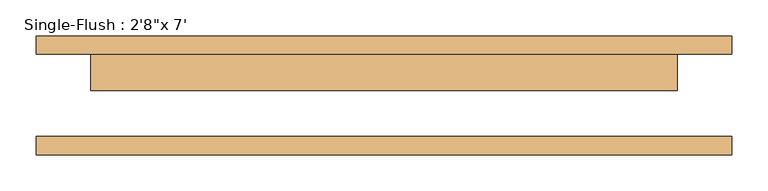
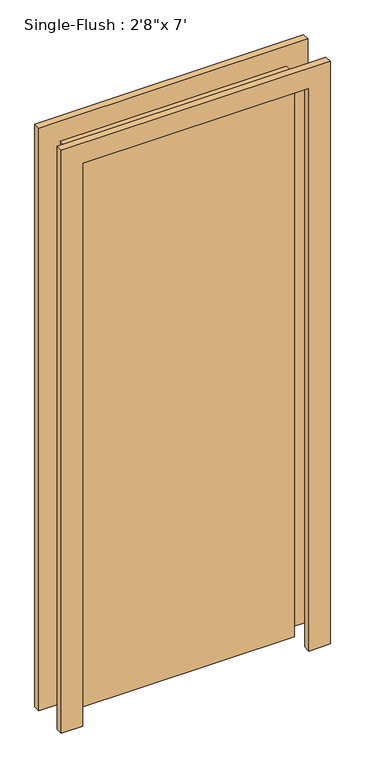
"""IFC4 building model written with IfcOpenShell, lengths in millimetres: door geometry."""

from ifc_helpers import new_model, si_unit, frame, origin, origin_with_axes, place, context, project, spatial, polyline, outline, extrude, source, transform, mapped, element, save


def door_d141acb4(model_context):
    return source(origin(), model_context, "Body", "SweptSolid", [
        extrude(outline(polyline([(2209.8, -482.6), (0.0, -482.6), (0.0, -406.4), (2133.6, -406.4), (2133.6, 406.4), (0.0, 406.4), (0.0, 482.6), (2209.8, 482.6), (2209.8, -482.6)])), frame((0.0, 57.15, 0.0), z_axis=(0.0, 1.0, 0.0), x_axis=(0.0, 0.0, 1.0)), (0.0, 0.0, 1.0), 25.4),
        extrude(outline(polyline([(2209.8, 482.6), (2209.8, -482.6), (0.0, -482.6), (0.0, -406.4), (2133.6, -406.4), (2133.6, 406.4), (0.0, 406.4), (0.0, 482.6), (2209.8, 482.6)])), frame((0.0, -82.55, 0.0), z_axis=(0.0, 1.0, 0.0), x_axis=(0.0, 0.0, 1.0)), (0.0, 0.0, 1.0), 25.4),
        extrude(outline(polyline([(406.4, 6.35), (-406.4, 6.35), (-406.4, 57.15), (406.4, 57.15), (406.4, 6.35)])), origin_with_axes(), (0.0, 0.0, 1.0), 2133.6),
    ])


if __name__ == "__main__":
    model = new_model("IFC4")
    model_context = context("Model", 3, world=origin())
    ifc_project = project(units=[si_unit("LENGTHUNIT", "METRE", prefix="MILLI")], contexts=[model_context])
    site = spatial("IfcSite", under=ifc_project)
    building = spatial("IfcBuilding", under=site)
    placement = place(None, origin())
    door_shape = door_d141acb4(model_context)
    element("IfcDoor", 1, ObjectType="Single-Flush : 2'8\"x 7'", at=placement, inside=building, context=model_context, shape_type="MappedRepresentation", body=[
        mapped(door_shape, transform((0.0, 0.0, 0.0), x_axis=(1.0, 0.0, 0.0), y_axis=(0.0, 1.0, 0.0), z_axis=(0.0, 0.0, 1.0))),
    ])
    save(model, "model.ifc")

# Revit data of these elements
# Type "Single-Flush : 2'8\"x 7'"
#   Type Mark = "11"
#   Construction Type Id = "MDOOR"
#   Assembly Code = "C1020"
#   Analytic Construction = "Metal"
#   Thickness = 0' - 2"
#   Heat Transfer Coefficient (U) = 0.651978 BTU/(h·ft²·°F)
#   Height = 7' - 0"
#   Trim Projection Ext = 0' - 1"
#   Trim Projection Int = 0' - 1"
#   Trim Width = 0' - 3"
#   Width = 2' - 8"
#   Define Thermal Properties by = 1
#   Door Material = Door - Panel
#   Frame Material = Door - Frame
#   Visual Light Transmittance = 0
#   Solar Heat Gain Coefficient = 0
#   Function = (empty or 0)
#   Wall Closure = (empty or 0)
# Element 1 (IfcDoor, "Single-Flush : 2'8\"x 7'")
#   Materials on its faces: "Door - Frame", "Door - Panel"
# Materials
#   "Door - Panel": class "Wood", colour RGB 210 159 95, transparency 0, Cost = 0
#   "Door - Frame": colour RGB 118 70 51, transparency 0, Cost = 0
